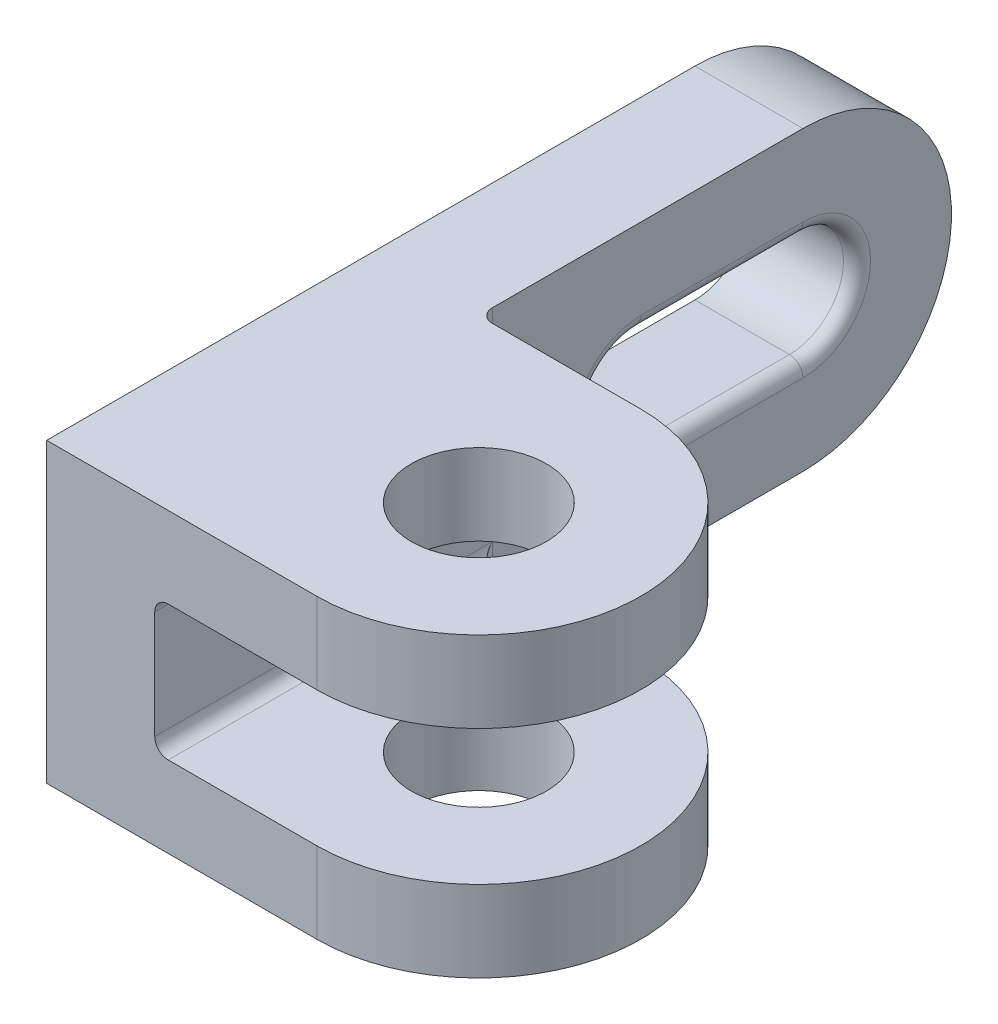
ISO-10303-21;
HEADER;
FILE_DESCRIPTION(('STEP AP214'),'2;1');
FILE_NAME('part.step','',(''),(''),'','','');
FILE_SCHEMA(('AUTOMOTIVE_DESIGN { 1 0 10303 214 1 1 1 1 }'));
ENDSEC;
DATA;
#1=APPLICATION_CONTEXT('core data for automotive mechanical design processes');
#2=APPLICATION_PROTOCOL_DEFINITION('international standard','automotive_design',2000,#1);
#3=PRODUCT_CONTEXT('',#1,'mechanical');
#4=PRODUCT('Part','Part','',(#3));
#5=PRODUCT_RELATED_PRODUCT_CATEGORY('part','',(#4));
#6=PRODUCT_DEFINITION_FORMATION('','',#4);
#7=PRODUCT_DEFINITION_CONTEXT('part definition',#1,'design');
#8=PRODUCT_DEFINITION('design','',#6,#7);
#9=PRODUCT_DEFINITION_SHAPE('','',#8);
#10=(LENGTH_UNIT() NAMED_UNIT(*) SI_UNIT(.MILLI.,.METRE.));
#11=(NAMED_UNIT(*) PLANE_ANGLE_UNIT() SI_UNIT($,.RADIAN.));
#12=(NAMED_UNIT(*) SI_UNIT($,.STERADIAN.) SOLID_ANGLE_UNIT());
#13=UNCERTAINTY_MEASURE_WITH_UNIT(LENGTH_MEASURE(1.E-05),#10,'distance_accuracy_value','');
#14=(GEOMETRIC_REPRESENTATION_CONTEXT(3) GLOBAL_UNCERTAINTY_ASSIGNED_CONTEXT((#13)) GLOBAL_UNIT_ASSIGNED_CONTEXT((#10,
#11,#12)) REPRESENTATION_CONTEXT('',''));
#15=CARTESIAN_POINT('',(0.,0.,0.));
#16=DIRECTION('',(0.,0.,1.));
#17=DIRECTION('',(1.,0.,0.));
#18=AXIS2_PLACEMENT_3D('',#15,#16,#17);
#19=CARTESIAN_POINT('',(16.,0.,-96.));
#20=DIRECTION('',(0.,1.,0.));
#21=DIRECTION('',(0.,0.,1.));
#22=AXIS2_PLACEMENT_3D('',#19,#20,#21);
#23=PLANE('',#22);
#24=CARTESIAN_POINT('',(40.,0.,-24.));
#25=DIRECTION('',(0.,-1.,0.));
#26=DIRECTION('',(0.,0.,-1.));
#27=AXIS2_PLACEMENT_3D('',#24,#25,#26);
#28=CIRCLE('',#27,10.);
#29=CARTESIAN_POINT('',(40.,0.,-34.));
#30=VERTEX_POINT('',#29);
#31=EDGE_CURVE('E308',#30,#30,#28,.T.);
#32=ORIENTED_EDGE('',*,*,#31,.F.);
#33=EDGE_LOOP('',(#32));
#34=FACE_BOUND('',#33,.T.);
#35=DIRECTION('',(0.,0.,-1.));
#36=VECTOR('',#35,1.);
#37=CARTESIAN_POINT('',(16.,0.,-96.));
#38=LINE('',#37,#36);
#39=CARTESIAN_POINT('',(16.,0.,-50.));
#40=VERTEX_POINT('',#39);
#41=CARTESIAN_POINT('',(16.,0.,-96.));
#42=VERTEX_POINT('',#41);
#43=EDGE_CURVE('E250',#40,#42,#38,.T.);
#44=ORIENTED_EDGE('',*,*,#43,.F.);
#45=CARTESIAN_POINT('',(18.,0.,-50.));
#46=DIRECTION('',(0.,1.,0.));
#47=DIRECTION('',(0.,0.,1.));
#48=AXIS2_PLACEMENT_3D('',#45,#46,#47);
#49=CIRCLE('',#48,2.);
#50=CARTESIAN_POINT('',(18.,0.,-48.));
#51=VERTEX_POINT('',#50);
#52=EDGE_CURVE('E282',#40,#51,#49,.T.);
#53=ORIENTED_EDGE('',*,*,#52,.T.);
#54=DIRECTION('',(1.,0.,0.));
#55=VECTOR('',#54,1.);
#56=CARTESIAN_POINT('',(40.,0.,-48.));
#57=LINE('',#56,#55);
#58=CARTESIAN_POINT('',(40.,0.,-48.));
#59=VERTEX_POINT('',#58);
#60=EDGE_CURVE('E202',#51,#59,#57,.T.);
#61=ORIENTED_EDGE('',*,*,#60,.T.);
#62=CARTESIAN_POINT('',(40.,0.,-24.));
#63=DIRECTION('',(0.,-1.,0.));
#64=DIRECTION('',(0.,0.,1.));
#65=AXIS2_PLACEMENT_3D('',#62,#63,#64);
#66=CIRCLE('',#65,24.);
#67=CARTESIAN_POINT('',(40.,0.,0.));
#68=VERTEX_POINT('',#67);
#69=EDGE_CURVE('E209',#59,#68,#66,.T.);
#70=ORIENTED_EDGE('',*,*,#69,.T.);
#71=DIRECTION('',(-1.,0.,0.));
#72=VECTOR('',#71,1.);
#73=CARTESIAN_POINT('',(16.,0.,0.));
#74=LINE('',#73,#72);
#75=CARTESIAN_POINT('',(0.,0.,0.));
#76=VERTEX_POINT('',#75);
#77=EDGE_CURVE('E256',#68,#76,#74,.T.);
#78=ORIENTED_EDGE('',*,*,#77,.T.);
#79=DIRECTION('',(0.,0.,-1.));
#80=VECTOR('',#79,1.);
#81=CARTESIAN_POINT('',(0.,0.,-96.));
#82=LINE('',#81,#80);
#83=CARTESIAN_POINT('',(0.,0.,-96.));
#84=VERTEX_POINT('',#83);
#85=EDGE_CURVE('E238',#76,#84,#82,.T.);
#86=ORIENTED_EDGE('',*,*,#85,.T.);
#87=DIRECTION('',(-1.,0.,0.));
#88=VECTOR('',#87,1.);
#89=CARTESIAN_POINT('',(16.,0.,-96.));
#90=LINE('',#89,#88);
#91=EDGE_CURVE('E275',#42,#84,#90,.T.);
#92=ORIENTED_EDGE('',*,*,#91,.F.);
#93=EDGE_LOOP('',(#44,#53,#61,#70,#78,#86,#92));
#94=FACE_BOUND('',#93,.T.);
#95=ADVANCED_FACE('F39',(#34,#94),#23,.F.);
#96=CARTESIAN_POINT('',(16.,22.,-96.));
#97=DIRECTION('',(-1.,0.,0.));
#98=DIRECTION('',(0.,0.,1.));
#99=AXIS2_PLACEMENT_3D('',#96,#97,#98);
#100=CYLINDRICAL_SURFACE('',#99,22.);
#101=CARTESIAN_POINT('',(0.,22.,-96.));
#102=DIRECTION('',(1.,0.,0.));
#103=DIRECTION('',(0.,0.,1.));
#104=AXIS2_PLACEMENT_3D('',#101,#102,#103);
#105=CIRCLE('',#104,22.);
#106=CARTESIAN_POINT('',(0.,44.,-96.));
#107=VERTEX_POINT('',#106);
#108=EDGE_CURVE('E257',#84,#107,#105,.T.);
#109=ORIENTED_EDGE('',*,*,#108,.T.);
#110=DIRECTION('',(-1.,0.,0.));
#111=VECTOR('',#110,1.);
#112=CARTESIAN_POINT('',(16.,44.,-96.));
#113=LINE('',#112,#111);
#114=CARTESIAN_POINT('',(16.,44.,-96.));
#115=VERTEX_POINT('',#114);
#116=EDGE_CURVE('E267',#115,#107,#113,.T.);
#117=ORIENTED_EDGE('',*,*,#116,.F.);
#118=CARTESIAN_POINT('',(16.,22.,-96.));
#119=DIRECTION('',(1.,0.,0.));
#120=DIRECTION('',(0.,0.,1.));
#121=AXIS2_PLACEMENT_3D('',#118,#119,#120);
#122=CIRCLE('',#121,22.);
#123=EDGE_CURVE('E247',#42,#115,#122,.T.);
#124=ORIENTED_EDGE('',*,*,#123,.F.);
#125=ORIENTED_EDGE('',*,*,#91,.T.);
#126=EDGE_LOOP('',(#109,#117,#124,#125));
#127=FACE_BOUND('',#126,.T.);
#128=ADVANCED_FACE('F375',(#127),#100,.T.);
#129=CARTESIAN_POINT('',(16.,44.,0.));
#130=DIRECTION('',(0.,-1.,0.));
#131=DIRECTION('',(0.,0.,-1.));
#132=AXIS2_PLACEMENT_3D('',#129,#130,#131);
#133=PLANE('',#132);
#134=CARTESIAN_POINT('',(40.,44.,-24.));
#135=DIRECTION('',(0.,1.,0.));
#136=DIRECTION('',(0.,0.,1.));
#137=AXIS2_PLACEMENT_3D('',#134,#135,#136);
#138=CIRCLE('',#137,10.);
#139=CARTESIAN_POINT('',(40.,44.,-14.));
#140=VERTEX_POINT('',#139);
#141=EDGE_CURVE('E608',#140,#140,#138,.T.);
#142=ORIENTED_EDGE('',*,*,#141,.F.);
#143=EDGE_LOOP('',(#142));
#144=FACE_BOUND('',#143,.T.);
#145=DIRECTION('',(0.,0.,1.));
#146=VECTOR('',#145,1.);
#147=CARTESIAN_POINT('',(0.,44.,0.));
#148=LINE('',#147,#146);
#149=CARTESIAN_POINT('',(0.,44.,0.));
#150=VERTEX_POINT('',#149);
#151=EDGE_CURVE('E265',#107,#150,#148,.T.);
#152=ORIENTED_EDGE('',*,*,#151,.T.);
#153=DIRECTION('',(-1.,0.,0.));
#154=VECTOR('',#153,1.);
#155=CARTESIAN_POINT('',(16.,44.,0.));
#156=LINE('',#155,#154);
#157=CARTESIAN_POINT('',(40.,44.,0.));
#158=VERTEX_POINT('',#157);
#159=EDGE_CURVE('E270',#158,#150,#156,.T.);
#160=ORIENTED_EDGE('',*,*,#159,.F.);
#161=CARTESIAN_POINT('',(40.,44.,-24.));
#162=DIRECTION('',(0.,1.,0.));
#163=DIRECTION('',(0.,0.,1.));
#164=AXIS2_PLACEMENT_3D('',#161,#162,#163);
#165=CIRCLE('',#164,24.);
#166=CARTESIAN_POINT('',(39.9999999999999,44.,-48.));
#167=VERTEX_POINT('',#166);
#168=EDGE_CURVE('E191',#158,#167,#165,.T.);
#169=ORIENTED_EDGE('',*,*,#168,.T.);
#170=DIRECTION('',(-1.,0.,0.));
#171=VECTOR('',#170,1.);
#172=CARTESIAN_POINT('',(39.9999999999999,44.,-48.));
#173=LINE('',#172,#171);
#174=CARTESIAN_POINT('',(18.,44.,-48.));
#175=VERTEX_POINT('',#174);
#176=EDGE_CURVE('E184',#167,#175,#173,.T.);
#177=ORIENTED_EDGE('',*,*,#176,.T.);
#178=CARTESIAN_POINT('',(18.,44.,-50.));
#179=DIRECTION('',(0.,-1.,0.));
#180=DIRECTION('',(0.,0.,-1.));
#181=AXIS2_PLACEMENT_3D('',#178,#179,#180);
#182=CIRCLE('',#181,2.);
#183=CARTESIAN_POINT('',(16.,44.,-50.));
#184=VERTEX_POINT('',#183);
#185=EDGE_CURVE('E301',#175,#184,#182,.T.);
#186=ORIENTED_EDGE('',*,*,#185,.T.);
#187=DIRECTION('',(0.,0.,1.));
#188=VECTOR('',#187,1.);
#189=CARTESIAN_POINT('',(16.,44.,0.));
#190=LINE('',#189,#188);
#191=EDGE_CURVE('E252',#115,#184,#190,.T.);
#192=ORIENTED_EDGE('',*,*,#191,.F.);
#193=ORIENTED_EDGE('',*,*,#116,.T.);
#194=EDGE_LOOP('',(#152,#160,#169,#177,#186,#192,#193));
#195=FACE_BOUND('',#194,.T.);
#196=ADVANCED_FACE('F379',(#144,#195),#133,.F.);
#197=CARTESIAN_POINT('',(16.,0.,0.));
#198=DIRECTION('',(0.,0.,-1.));
#199=DIRECTION('',(-1.,0.,0.));
#200=AXIS2_PLACEMENT_3D('',#197,#198,#199);
#201=PLANE('',#200);
#202=DIRECTION('',(0.,-1.,0.));
#203=VECTOR('',#202,1.);
#204=CARTESIAN_POINT('',(0.,0.,0.));
#205=LINE('',#204,#203);
#206=EDGE_CURVE('E249',#150,#76,#205,.T.);
#207=ORIENTED_EDGE('',*,*,#206,.T.);
#208=ORIENTED_EDGE('',*,*,#77,.F.);
#209=DIRECTION('',(0.,-1.,0.));
#210=VECTOR('',#209,1.);
#211=CARTESIAN_POINT('',(40.,12.,0.));
#212=LINE('',#211,#210);
#213=CARTESIAN_POINT('',(40.,12.,0.));
#214=VERTEX_POINT('',#213);
#215=EDGE_CURVE('E219',#214,#68,#212,.T.);
#216=ORIENTED_EDGE('',*,*,#215,.F.);
#217=DIRECTION('',(-1.,0.,0.));
#218=VECTOR('',#217,1.);
#219=CARTESIAN_POINT('',(0.,12.,0.));
#220=LINE('',#219,#218);
#221=CARTESIAN_POINT('',(18.,12.,0.));
#222=VERTEX_POINT('',#221);
#223=EDGE_CURVE('E213',#214,#222,#220,.T.);
#224=ORIENTED_EDGE('',*,*,#223,.T.);
#225=CARTESIAN_POINT('',(18.,14.,0.));
#226=DIRECTION('',(0.,0.,-1.));
#227=DIRECTION('',(-1.,0.,0.));
#228=AXIS2_PLACEMENT_3D('',#225,#226,#227);
#229=CIRCLE('',#228,2.);
#230=CARTESIAN_POINT('',(16.,14.,0.));
#231=VERTEX_POINT('',#230);
#232=EDGE_CURVE('E298',#222,#231,#229,.T.);
#233=ORIENTED_EDGE('',*,*,#232,.T.);
#234=DIRECTION('',(0.,-1.,0.));
#235=VECTOR('',#234,1.);
#236=CARTESIAN_POINT('',(16.,0.,0.));
#237=LINE('',#236,#235);
#238=CARTESIAN_POINT('',(16.,30.,0.));
#239=VERTEX_POINT('',#238);
#240=EDGE_CURVE('E254',#239,#231,#237,.T.);
#241=ORIENTED_EDGE('',*,*,#240,.F.);
#242=CARTESIAN_POINT('',(18.,30.,0.));
#243=DIRECTION('',(0.,0.,-1.));
#244=DIRECTION('',(-1.,0.,0.));
#245=AXIS2_PLACEMENT_3D('',#242,#243,#244);
#246=CIRCLE('',#245,2.);
#247=CARTESIAN_POINT('',(18.,32.,0.));
#248=VERTEX_POINT('',#247);
#249=EDGE_CURVE('E178',#239,#248,#246,.T.);
#250=ORIENTED_EDGE('',*,*,#249,.T.);
#251=DIRECTION('',(1.,0.,0.));
#252=VECTOR('',#251,1.);
#253=CARTESIAN_POINT('',(0.,32.,0.));
#254=LINE('',#253,#252);
#255=CARTESIAN_POINT('',(40.,32.,0.));
#256=VERTEX_POINT('',#255);
#257=EDGE_CURVE('E168',#248,#256,#254,.T.);
#258=ORIENTED_EDGE('',*,*,#257,.T.);
#259=DIRECTION('',(0.,1.,0.));
#260=VECTOR('',#259,1.);
#261=CARTESIAN_POINT('',(40.,32.,0.));
#262=LINE('',#261,#260);
#263=EDGE_CURVE('E174',#256,#158,#262,.T.);
#264=ORIENTED_EDGE('',*,*,#263,.T.);
#265=ORIENTED_EDGE('',*,*,#159,.T.);
#266=EDGE_LOOP('',(#207,#208,#216,#224,#233,#241,#250,#258,#264,#265));
#267=FACE_BOUND('',#266,.T.);
#268=ADVANCED_FACE('F175',(#267),#201,.F.);
#269=CARTESIAN_POINT('',(16.,22.,-96.));
#270=DIRECTION('',(-1.,0.,0.));
#271=DIRECTION('',(0.,0.,1.));
#272=AXIS2_PLACEMENT_3D('',#269,#270,#271);
#273=PLANE('',#272);
#274=DIRECTION('',(0.,0.,1.));
#275=VECTOR('',#274,1.);
#276=CARTESIAN_POINT('',(16.,32.,-96.));
#277=LINE('',#276,#275);
#278=CARTESIAN_POINT('',(16.,32.,-72.));
#279=VERTEX_POINT('',#278);
#280=CARTESIAN_POINT('',(16.,32.,-96.));
#281=VERTEX_POINT('',#280);
#282=EDGE_CURVE('E310',#279,#281,#277,.F.);
#283=ORIENTED_EDGE('',*,*,#282,.T.);
#284=CARTESIAN_POINT('',(16.,22.,-96.));
#285=DIRECTION('',(-1.,0.,0.));
#286=DIRECTION('',(0.,0.,1.));
#287=AXIS2_PLACEMENT_3D('',#284,#285,#286);
#288=CIRCLE('',#287,10.);
#289=CARTESIAN_POINT('',(16.,12.,-96.));
#290=VERTEX_POINT('',#289);
#291=EDGE_CURVE('E312',#281,#290,#288,.T.);
#292=ORIENTED_EDGE('',*,*,#291,.T.);
#293=DIRECTION('',(0.,0.,-1.));
#294=VECTOR('',#293,1.);
#295=CARTESIAN_POINT('',(16.,12.,-96.));
#296=LINE('',#295,#294);
#297=CARTESIAN_POINT('',(16.,12.,-72.));
#298=VERTEX_POINT('',#297);
#299=EDGE_CURVE('E311',#290,#298,#296,.F.);
#300=ORIENTED_EDGE('',*,*,#299,.T.);
#301=CARTESIAN_POINT('',(16.,22.,-72.));
#302=DIRECTION('',(-1.,0.,0.));
#303=DIRECTION('',(0.,0.,1.));
#304=AXIS2_PLACEMENT_3D('',#301,#302,#303);
#305=CIRCLE('',#304,10.);
#306=EDGE_CURVE('E313',#298,#279,#305,.T.);
#307=ORIENTED_EDGE('',*,*,#306,.T.);
#308=EDGE_LOOP('',(#283,#292,#300,#307));
#309=FACE_BOUND('',#308,.T.);
#310=ORIENTED_EDGE('',*,*,#240,.T.);
#311=DIRECTION('',(0.,0.,-1.));
#312=VECTOR('',#311,1.);
#313=CARTESIAN_POINT('',(16.,14.,-96.));
#314=LINE('',#313,#312);
#315=CARTESIAN_POINT('',(16.,14.,-50.));
#316=VERTEX_POINT('',#315);
#317=EDGE_CURVE('E290',#231,#316,#314,.T.);
#318=ORIENTED_EDGE('',*,*,#317,.T.);
#319=DIRECTION('',(0.,-1.,0.));
#320=VECTOR('',#319,1.);
#321=CARTESIAN_POINT('',(16.,22.,-50.));
#322=LINE('',#321,#320);
#323=EDGE_CURVE('E274',#316,#40,#322,.T.);
#324=ORIENTED_EDGE('',*,*,#323,.T.);
#325=ORIENTED_EDGE('',*,*,#43,.T.);
#326=ORIENTED_EDGE('',*,*,#123,.T.);
#327=ORIENTED_EDGE('',*,*,#191,.T.);
#328=DIRECTION('',(0.,-1.,0.));
#329=VECTOR('',#328,1.);
#330=CARTESIAN_POINT('',(16.,22.,-50.));
#331=LINE('',#330,#329);
#332=CARTESIAN_POINT('',(16.,30.,-50.));
#333=VERTEX_POINT('',#332);
#334=EDGE_CURVE('E283',#184,#333,#331,.T.);
#335=ORIENTED_EDGE('',*,*,#334,.T.);
#336=DIRECTION('',(0.,0.,-1.));
#337=VECTOR('',#336,1.);
#338=CARTESIAN_POINT('',(16.,30.,0.));
#339=LINE('',#338,#337);
#340=EDGE_CURVE('E281',#333,#239,#339,.F.);
#341=ORIENTED_EDGE('',*,*,#340,.T.);
#342=EDGE_LOOP('',(#310,#318,#324,#325,#326,#327,#335,#341));
#343=FACE_BOUND('',#342,.T.);
#344=ADVANCED_FACE('F339',(#309,#343),#273,.F.);
#345=CARTESIAN_POINT('',(0.,22.,-96.));
#346=DIRECTION('',(-1.,0.,0.));
#347=DIRECTION('',(0.,0.,1.));
#348=AXIS2_PLACEMENT_3D('',#345,#346,#347);
#349=PLANE('',#348);
#350=ORIENTED_EDGE('',*,*,#206,.F.);
#351=ORIENTED_EDGE('',*,*,#151,.F.);
#352=ORIENTED_EDGE('',*,*,#108,.F.);
#353=ORIENTED_EDGE('',*,*,#85,.F.);
#354=EDGE_LOOP('',(#350,#351,#352,#353));
#355=FACE_BOUND('',#354,.T.);
#356=CARTESIAN_POINT('',(0.,22.,-72.));
#357=DIRECTION('',(1.,0.,0.));
#358=DIRECTION('',(0.,0.,-1.));
#359=AXIS2_PLACEMENT_3D('',#356,#357,#358);
#360=CIRCLE('',#359,8.00000000000001);
#361=CARTESIAN_POINT('',(0.,30.,-72.));
#362=VERTEX_POINT('',#361);
#363=CARTESIAN_POINT('',(0.,14.,-72.));
#364=VERTEX_POINT('',#363);
#365=EDGE_CURVE('E224',#362,#364,#360,.T.);
#366=ORIENTED_EDGE('',*,*,#365,.T.);
#367=DIRECTION('',(0.,0.,-1.));
#368=VECTOR('',#367,1.);
#369=CARTESIAN_POINT('',(0.,14.,-96.));
#370=LINE('',#369,#368);
#371=CARTESIAN_POINT('',(0.,14.,-96.));
#372=VERTEX_POINT('',#371);
#373=EDGE_CURVE('E228',#364,#372,#370,.T.);
#374=ORIENTED_EDGE('',*,*,#373,.T.);
#375=CARTESIAN_POINT('',(0.,22.,-96.));
#376=DIRECTION('',(1.,0.,0.));
#377=DIRECTION('',(0.,0.,-1.));
#378=AXIS2_PLACEMENT_3D('',#375,#376,#377);
#379=CIRCLE('',#378,8.00000000000001);
#380=CARTESIAN_POINT('',(0.,30.,-96.));
#381=VERTEX_POINT('',#380);
#382=EDGE_CURVE('E231',#372,#381,#379,.T.);
#383=ORIENTED_EDGE('',*,*,#382,.T.);
#384=DIRECTION('',(0.,0.,1.));
#385=VECTOR('',#384,1.);
#386=CARTESIAN_POINT('',(0.,30.,-72.));
#387=LINE('',#386,#385);
#388=EDGE_CURVE('E232',#381,#362,#387,.T.);
#389=ORIENTED_EDGE('',*,*,#388,.T.);
#390=EDGE_LOOP('',(#366,#374,#383,#389));
#391=FACE_BOUND('',#390,.T.);
#392=ADVANCED_FACE('F354',(#355,#391),#349,.T.);
#393=CARTESIAN_POINT('',(0.,22.,-72.));
#394=DIRECTION('',(1.,0.,0.));
#395=DIRECTION('',(0.,0.,-1.));
#396=AXIS2_PLACEMENT_3D('',#393,#394,#395);
#397=CYLINDRICAL_SURFACE('',#396,8.00000000000001);
#398=DIRECTION('',(1.,0.,0.));
#399=VECTOR('',#398,1.);
#400=CARTESIAN_POINT('',(0.,30.,-72.));
#401=LINE('',#400,#399);
#402=CARTESIAN_POINT('',(14.,30.,-72.));
#403=VERTEX_POINT('',#402);
#404=EDGE_CURVE('E236',#362,#403,#401,.T.);
#405=ORIENTED_EDGE('',*,*,#404,.T.);
#406=CARTESIAN_POINT('',(14.,22.,-72.));
#407=DIRECTION('',(-1.,0.,0.));
#408=DIRECTION('',(0.,0.,1.));
#409=AXIS2_PLACEMENT_3D('',#406,#407,#408);
#410=CIRCLE('',#409,8.00000000000001);
#411=CARTESIAN_POINT('',(14.,14.,-72.));
#412=VERTEX_POINT('',#411);
#413=EDGE_CURVE('E48',#403,#412,#410,.F.);
#414=ORIENTED_EDGE('',*,*,#413,.T.);
#415=DIRECTION('',(1.,0.,0.));
#416=VECTOR('',#415,1.);
#417=CARTESIAN_POINT('',(0.,14.,-72.));
#418=LINE('',#417,#416);
#419=EDGE_CURVE('E240',#364,#412,#418,.T.);
#420=ORIENTED_EDGE('',*,*,#419,.F.);
#421=ORIENTED_EDGE('',*,*,#365,.F.);
#422=EDGE_LOOP('',(#405,#414,#420,#421));
#423=FACE_BOUND('',#422,.T.);
#424=ADVANCED_FACE('F358',(#423),#397,.F.);
#425=CARTESIAN_POINT('',(0.,30.,-72.));
#426=DIRECTION('',(0.,1.,0.));
#427=DIRECTION('',(0.,0.,1.));
#428=AXIS2_PLACEMENT_3D('',#425,#426,#427);
#429=PLANE('',#428);
#430=DIRECTION('',(1.,0.,0.));
#431=VECTOR('',#430,1.);
#432=CARTESIAN_POINT('',(0.,30.,-96.));
#433=LINE('',#432,#431);
#434=CARTESIAN_POINT('',(14.,30.,-96.));
#435=VERTEX_POINT('',#434);
#436=EDGE_CURVE('E242',#381,#435,#433,.T.);
#437=ORIENTED_EDGE('',*,*,#436,.T.);
#438=DIRECTION('',(0.,0.,1.));
#439=VECTOR('',#438,1.);
#440=CARTESIAN_POINT('',(14.,30.,-72.));
#441=LINE('',#440,#439);
#442=EDGE_CURVE('E11',#435,#403,#441,.T.);
#443=ORIENTED_EDGE('',*,*,#442,.T.);
#444=ORIENTED_EDGE('',*,*,#404,.F.);
#445=ORIENTED_EDGE('',*,*,#388,.F.);
#446=EDGE_LOOP('',(#437,#443,#444,#445));
#447=FACE_BOUND('',#446,.T.);
#448=ADVANCED_FACE('F352',(#447),#429,.F.);
#449=CARTESIAN_POINT('',(0.,22.,-96.));
#450=DIRECTION('',(1.,0.,0.));
#451=DIRECTION('',(0.,0.,-1.));
#452=AXIS2_PLACEMENT_3D('',#449,#450,#451);
#453=CYLINDRICAL_SURFACE('',#452,8.00000000000001);
#454=DIRECTION('',(1.,0.,0.));
#455=VECTOR('',#454,1.);
#456=CARTESIAN_POINT('',(0.,14.,-96.));
#457=LINE('',#456,#455);
#458=CARTESIAN_POINT('',(14.,14.,-96.));
#459=VERTEX_POINT('',#458);
#460=EDGE_CURVE('E243',#372,#459,#457,.T.);
#461=ORIENTED_EDGE('',*,*,#460,.T.);
#462=CARTESIAN_POINT('',(14.,22.,-96.));
#463=DIRECTION('',(-1.,0.,0.));
#464=DIRECTION('',(0.,0.,1.));
#465=AXIS2_PLACEMENT_3D('',#462,#463,#464);
#466=CIRCLE('',#465,8.00000000000001);
#467=EDGE_CURVE('E303',#459,#435,#466,.F.);
#468=ORIENTED_EDGE('',*,*,#467,.T.);
#469=ORIENTED_EDGE('',*,*,#436,.F.);
#470=ORIENTED_EDGE('',*,*,#382,.F.);
#471=EDGE_LOOP('',(#461,#468,#469,#470));
#472=FACE_BOUND('',#471,.T.);
#473=ADVANCED_FACE('F346',(#472),#453,.F.);
#474=CARTESIAN_POINT('',(0.,14.,-96.));
#475=DIRECTION('',(0.,-1.,0.));
#476=DIRECTION('',(0.,0.,-1.));
#477=AXIS2_PLACEMENT_3D('',#474,#475,#476);
#478=PLANE('',#477);
#479=ORIENTED_EDGE('',*,*,#419,.T.);
#480=DIRECTION('',(0.,0.,-1.));
#481=VECTOR('',#480,1.);
#482=CARTESIAN_POINT('',(14.,14.,-96.));
#483=LINE('',#482,#481);
#484=EDGE_CURVE('E318',#412,#459,#483,.T.);
#485=ORIENTED_EDGE('',*,*,#484,.T.);
#486=ORIENTED_EDGE('',*,*,#460,.F.);
#487=ORIENTED_EDGE('',*,*,#373,.F.);
#488=EDGE_LOOP('',(#479,#485,#486,#487));
#489=FACE_BOUND('',#488,.T.);
#490=ADVANCED_FACE('F360',(#489),#478,.F.);
#491=CARTESIAN_POINT('',(40.,12.,-48.));
#492=DIRECTION('',(0.,0.,-1.));
#493=DIRECTION('',(-1.,0.,0.));
#494=AXIS2_PLACEMENT_3D('',#491,#492,#493);
#495=PLANE('',#494);
#496=ORIENTED_EDGE('',*,*,#60,.F.);
#497=DIRECTION('',(0.,-1.,0.));
#498=VECTOR('',#497,1.);
#499=CARTESIAN_POINT('',(18.,12.,-48.));
#500=LINE('',#499,#498);
#501=CARTESIAN_POINT('',(18.,12.,-48.));
#502=VERTEX_POINT('',#501);
#503=EDGE_CURVE('E279',#51,#502,#500,.F.);
#504=ORIENTED_EDGE('',*,*,#503,.T.);
#505=DIRECTION('',(1.,0.,0.));
#506=VECTOR('',#505,1.);
#507=CARTESIAN_POINT('',(40.,12.,-48.));
#508=LINE('',#507,#506);
#509=CARTESIAN_POINT('',(40.,12.,-48.));
#510=VERTEX_POINT('',#509);
#511=EDGE_CURVE('E210',#502,#510,#508,.T.);
#512=ORIENTED_EDGE('',*,*,#511,.T.);
#513=DIRECTION('',(0.,-1.,0.));
#514=VECTOR('',#513,1.);
#515=CARTESIAN_POINT('',(40.,12.,-48.));
#516=LINE('',#515,#514);
#517=EDGE_CURVE('E216',#510,#59,#516,.T.);
#518=ORIENTED_EDGE('',*,*,#517,.T.);
#519=EDGE_LOOP('',(#496,#504,#512,#518));
#520=FACE_BOUND('',#519,.T.);
#521=ADVANCED_FACE('F423',(#520),#495,.T.);
#522=CARTESIAN_POINT('',(40.,12.,-24.));
#523=DIRECTION('',(0.,1.,0.));
#524=DIRECTION('',(0.,0.,1.));
#525=AXIS2_PLACEMENT_3D('',#522,#523,#524);
#526=PLANE('',#525);
#527=CARTESIAN_POINT('',(40.,12.,-24.));
#528=DIRECTION('',(0.,-1.,0.));
#529=DIRECTION('',(0.,0.,-1.));
#530=AXIS2_PLACEMENT_3D('',#527,#528,#529);
#531=CIRCLE('',#530,10.);
#532=CARTESIAN_POINT('',(40.,12.,-34.));
#533=VERTEX_POINT('',#532);
#534=EDGE_CURVE('E610',#533,#533,#531,.T.);
#535=ORIENTED_EDGE('',*,*,#534,.T.);
#536=EDGE_LOOP('',(#535));
#537=FACE_BOUND('',#536,.T.);
#538=ORIENTED_EDGE('',*,*,#511,.F.);
#539=DIRECTION('',(0.,0.,-1.));
#540=VECTOR('',#539,1.);
#541=CARTESIAN_POINT('',(18.,12.,-24.));
#542=LINE('',#541,#540);
#543=EDGE_CURVE('E289',#502,#222,#542,.F.);
#544=ORIENTED_EDGE('',*,*,#543,.T.);
#545=ORIENTED_EDGE('',*,*,#223,.F.);
#546=CARTESIAN_POINT('',(40.,12.,-24.));
#547=DIRECTION('',(0.,-1.,0.));
#548=DIRECTION('',(0.,0.,1.));
#549=AXIS2_PLACEMENT_3D('',#546,#547,#548);
#550=CIRCLE('',#549,24.);
#551=EDGE_CURVE('E207',#510,#214,#550,.T.);
#552=ORIENTED_EDGE('',*,*,#551,.F.);
#553=EDGE_LOOP('',(#538,#544,#545,#552));
#554=FACE_BOUND('',#553,.T.);
#555=ADVANCED_FACE('F492',(#537,#554),#526,.T.);
#556=CARTESIAN_POINT('',(40.,12.,-24.));
#557=DIRECTION('',(0.,-1.,0.));
#558=DIRECTION('',(0.,0.,-1.));
#559=AXIS2_PLACEMENT_3D('',#556,#557,#558);
#560=CYLINDRICAL_SURFACE('',#559,24.);
#561=ORIENTED_EDGE('',*,*,#69,.F.);
#562=ORIENTED_EDGE('',*,*,#517,.F.);
#563=ORIENTED_EDGE('',*,*,#551,.T.);
#564=ORIENTED_EDGE('',*,*,#215,.T.);
#565=EDGE_LOOP('',(#561,#562,#563,#564));
#566=FACE_BOUND('',#565,.T.);
#567=ADVANCED_FACE('F489',(#566),#560,.T.);
#568=CARTESIAN_POINT('',(39.9999999999999,32.,-48.));
#569=DIRECTION('',(0.,0.,-1.));
#570=DIRECTION('',(-1.,0.,0.));
#571=AXIS2_PLACEMENT_3D('',#568,#569,#570);
#572=PLANE('',#571);
#573=DIRECTION('',(-1.,0.,0.));
#574=VECTOR('',#573,1.);
#575=CARTESIAN_POINT('',(39.9999999999999,32.,-48.));
#576=LINE('',#575,#574);
#577=CARTESIAN_POINT('',(39.9999999999999,32.,-48.));
#578=VERTEX_POINT('',#577);
#579=CARTESIAN_POINT('',(18.,32.,-48.));
#580=VERTEX_POINT('',#579);
#581=EDGE_CURVE('E193',#578,#580,#576,.T.);
#582=ORIENTED_EDGE('',*,*,#581,.T.);
#583=DIRECTION('',(0.,-1.,0.));
#584=VECTOR('',#583,1.);
#585=CARTESIAN_POINT('',(18.,32.,-48.));
#586=LINE('',#585,#584);
#587=EDGE_CURVE('E294',#580,#175,#586,.F.);
#588=ORIENTED_EDGE('',*,*,#587,.T.);
#589=ORIENTED_EDGE('',*,*,#176,.F.);
#590=DIRECTION('',(0.,1.,0.));
#591=VECTOR('',#590,1.);
#592=CARTESIAN_POINT('',(39.9999999999999,32.,-48.));
#593=LINE('',#592,#591);
#594=EDGE_CURVE('E195',#578,#167,#593,.T.);
#595=ORIENTED_EDGE('',*,*,#594,.F.);
#596=EDGE_LOOP('',(#582,#588,#589,#595));
#597=FACE_BOUND('',#596,.T.);
#598=ADVANCED_FACE('F495',(#597),#572,.T.);
#599=CARTESIAN_POINT('',(40.,32.,-24.));
#600=DIRECTION('',(0.,1.,0.));
#601=DIRECTION('',(0.,0.,1.));
#602=AXIS2_PLACEMENT_3D('',#599,#600,#601);
#603=PLANE('',#602);
#604=CARTESIAN_POINT('',(40.,32.,-24.));
#605=DIRECTION('',(0.,1.,0.));
#606=DIRECTION('',(0.,0.,1.));
#607=AXIS2_PLACEMENT_3D('',#604,#605,#606);
#608=CIRCLE('',#607,10.);
#609=CARTESIAN_POINT('',(40.,32.,-14.));
#610=VERTEX_POINT('',#609);
#611=EDGE_CURVE('E205',#610,#610,#608,.T.);
#612=ORIENTED_EDGE('',*,*,#611,.T.);
#613=EDGE_LOOP('',(#612));
#614=FACE_BOUND('',#613,.T.);
#615=ORIENTED_EDGE('',*,*,#257,.F.);
#616=DIRECTION('',(0.,0.,-1.));
#617=VECTOR('',#616,1.);
#618=CARTESIAN_POINT('',(18.,32.,-48.));
#619=LINE('',#618,#617);
#620=EDGE_CURVE('E295',#248,#580,#619,.T.);
#621=ORIENTED_EDGE('',*,*,#620,.T.);
#622=ORIENTED_EDGE('',*,*,#581,.F.);
#623=CARTESIAN_POINT('',(40.,32.,-24.));
#624=DIRECTION('',(0.,1.,0.));
#625=DIRECTION('',(0.,0.,1.));
#626=AXIS2_PLACEMENT_3D('',#623,#624,#625);
#627=CIRCLE('',#626,24.);
#628=EDGE_CURVE('E181',#256,#578,#627,.T.);
#629=ORIENTED_EDGE('',*,*,#628,.F.);
#630=EDGE_LOOP('',(#615,#621,#622,#629));
#631=FACE_BOUND('',#630,.T.);
#632=ADVANCED_FACE('F194',(#614,#631),#603,.F.);
#633=CARTESIAN_POINT('',(40.,32.,-24.));
#634=DIRECTION('',(0.,1.,0.));
#635=DIRECTION('',(0.,0.,1.));
#636=AXIS2_PLACEMENT_3D('',#633,#634,#635);
#637=CYLINDRICAL_SURFACE('',#636,24.);
#638=ORIENTED_EDGE('',*,*,#168,.F.);
#639=ORIENTED_EDGE('',*,*,#263,.F.);
#640=ORIENTED_EDGE('',*,*,#628,.T.);
#641=ORIENTED_EDGE('',*,*,#594,.T.);
#642=EDGE_LOOP('',(#638,#639,#640,#641));
#643=FACE_BOUND('',#642,.T.);
#644=ADVANCED_FACE('F188',(#643),#637,.T.);
#645=CARTESIAN_POINT('',(40.,32.,-24.));
#646=DIRECTION('',(0.,1.,0.));
#647=DIRECTION('',(0.,0.,1.));
#648=AXIS2_PLACEMENT_3D('',#645,#646,#647);
#649=CYLINDRICAL_SURFACE('',#648,10.);
#650=ORIENTED_EDGE('',*,*,#611,.F.);
#651=EDGE_LOOP('',(#650));
#652=FACE_BOUND('',#651,.T.);
#653=ORIENTED_EDGE('',*,*,#141,.T.);
#654=EDGE_LOOP('',(#653));
#655=FACE_BOUND('',#654,.T.);
#656=ADVANCED_FACE('F542',(#652,#655),#649,.F.);
#657=CARTESIAN_POINT('',(40.,12.,-24.));
#658=DIRECTION('',(0.,-1.,0.));
#659=DIRECTION('',(0.,0.,-1.));
#660=AXIS2_PLACEMENT_3D('',#657,#658,#659);
#661=CYLINDRICAL_SURFACE('',#660,10.);
#662=ORIENTED_EDGE('',*,*,#534,.F.);
#663=EDGE_LOOP('',(#662));
#664=FACE_BOUND('',#663,.T.);
#665=ORIENTED_EDGE('',*,*,#31,.T.);
#666=EDGE_LOOP('',(#665));
#667=FACE_BOUND('',#666,.T.);
#668=ADVANCED_FACE('F392',(#664,#667),#661,.F.);
#669=CARTESIAN_POINT('',(18.,22.,-50.));
#670=DIRECTION('',(0.,-1.,0.));
#671=DIRECTION('',(0.,0.,-1.));
#672=AXIS2_PLACEMENT_3D('',#669,#670,#671);
#673=CYLINDRICAL_SURFACE('',#672,2.);
#674=ORIENTED_EDGE('',*,*,#323,.F.);
#675=CARTESIAN_POINT('',(18.,14.,-50.));
#676=DIRECTION('',(0.,-0.707106781186547,-0.707106781186547));
#677=DIRECTION('',(0.,-0.707106781186547,0.707106781186547));
#678=AXIS2_PLACEMENT_3D('',#675,#676,#677);
#679=ELLIPSE('',#678,2.82842712474619,2.);
#680=EDGE_CURVE('E297',#316,#502,#679,.F.);
#681=ORIENTED_EDGE('',*,*,#680,.T.);
#682=ORIENTED_EDGE('',*,*,#503,.F.);
#683=ORIENTED_EDGE('',*,*,#52,.F.);
#684=EDGE_LOOP('',(#674,#681,#682,#683));
#685=FACE_BOUND('',#684,.T.);
#686=ADVANCED_FACE('F390',(#685),#673,.F.);
#687=CARTESIAN_POINT('',(18.,14.,-96.));
#688=DIRECTION('',(0.,0.,-1.));
#689=DIRECTION('',(0.,1.,0.));
#690=AXIS2_PLACEMENT_3D('',#687,#688,#689);
#691=CYLINDRICAL_SURFACE('',#690,2.);
#692=ORIENTED_EDGE('',*,*,#232,.F.);
#693=ORIENTED_EDGE('',*,*,#543,.F.);
#694=ORIENTED_EDGE('',*,*,#680,.F.);
#695=ORIENTED_EDGE('',*,*,#317,.F.);
#696=EDGE_LOOP('',(#692,#693,#694,#695));
#697=FACE_BOUND('',#696,.T.);
#698=ADVANCED_FACE('F388',(#697),#691,.F.);
#699=CARTESIAN_POINT('',(18.,22.,-50.));
#700=DIRECTION('',(0.,-1.,0.));
#701=DIRECTION('',(0.,0.,-1.));
#702=AXIS2_PLACEMENT_3D('',#699,#700,#701);
#703=CYLINDRICAL_SURFACE('',#702,2.);
#704=ORIENTED_EDGE('',*,*,#185,.F.);
#705=ORIENTED_EDGE('',*,*,#587,.F.);
#706=CARTESIAN_POINT('',(18.,30.,-50.));
#707=DIRECTION('',(0.,-0.707106781186547,0.707106781186547));
#708=DIRECTION('',(0.,-0.707106781186547,-0.707106781186547));
#709=AXIS2_PLACEMENT_3D('',#706,#707,#708);
#710=ELLIPSE('',#709,2.82842712474619,2.);
#711=EDGE_CURVE('E302',#333,#580,#710,.F.);
#712=ORIENTED_EDGE('',*,*,#711,.F.);
#713=ORIENTED_EDGE('',*,*,#334,.F.);
#714=EDGE_LOOP('',(#704,#705,#712,#713));
#715=FACE_BOUND('',#714,.T.);
#716=ADVANCED_FACE('F391',(#715),#703,.F.);
#717=CARTESIAN_POINT('',(18.,30.,-24.));
#718=DIRECTION('',(0.,0.,1.));
#719=DIRECTION('',(1.,0.,0.));
#720=AXIS2_PLACEMENT_3D('',#717,#718,#719);
#721=CYLINDRICAL_SURFACE('',#720,2.);
#722=ORIENTED_EDGE('',*,*,#249,.F.);
#723=ORIENTED_EDGE('',*,*,#340,.F.);
#724=ORIENTED_EDGE('',*,*,#711,.T.);
#725=ORIENTED_EDGE('',*,*,#620,.F.);
#726=EDGE_LOOP('',(#722,#723,#724,#725));
#727=FACE_BOUND('',#726,.T.);
#728=ADVANCED_FACE('F400',(#727),#721,.F.);
#729=CARTESIAN_POINT('',(14.,22.,-72.));
#730=DIRECTION('',(-1.,0.,0.));
#731=DIRECTION('',(0.,0.,1.));
#732=AXIS2_PLACEMENT_3D('',#729,#730,#731);
#733=TOROIDAL_SURFACE('',#732,10.,2.);
#734=CARTESIAN_POINT('',(14.,32.,-72.));
#735=DIRECTION('',(0.,0.,-1.));
#736=DIRECTION('',(-1.,0.,0.));
#737=AXIS2_PLACEMENT_3D('',#734,#735,#736);
#738=CIRCLE('',#737,2.);
#739=EDGE_CURVE('E322',#279,#403,#738,.T.);
#740=ORIENTED_EDGE('',*,*,#739,.F.);
#741=ORIENTED_EDGE('',*,*,#306,.F.);
#742=CARTESIAN_POINT('',(14.,12.,-72.));
#743=DIRECTION('',(0.,0.,-1.));
#744=DIRECTION('',(-1.,0.,0.));
#745=AXIS2_PLACEMENT_3D('',#742,#743,#744);
#746=CIRCLE('',#745,2.);
#747=EDGE_CURVE('E43',#412,#298,#746,.T.);
#748=ORIENTED_EDGE('',*,*,#747,.F.);
#749=ORIENTED_EDGE('',*,*,#413,.F.);
#750=EDGE_LOOP('',(#740,#741,#748,#749));
#751=FACE_BOUND('',#750,.T.);
#752=ADVANCED_FACE('F41',(#751),#733,.T.);
#753=CARTESIAN_POINT('',(14.,12.,-96.));
#754=DIRECTION('',(0.,0.,-1.));
#755=DIRECTION('',(-1.,0.,0.));
#756=AXIS2_PLACEMENT_3D('',#753,#754,#755);
#757=CYLINDRICAL_SURFACE('',#756,2.);
#758=ORIENTED_EDGE('',*,*,#747,.T.);
#759=ORIENTED_EDGE('',*,*,#299,.F.);
#760=CARTESIAN_POINT('',(14.,12.,-96.));
#761=DIRECTION('',(0.,0.,-1.));
#762=DIRECTION('',(-1.,0.,0.));
#763=AXIS2_PLACEMENT_3D('',#760,#761,#762);
#764=CIRCLE('',#763,2.);
#765=EDGE_CURVE('E323',#459,#290,#764,.T.);
#766=ORIENTED_EDGE('',*,*,#765,.F.);
#767=ORIENTED_EDGE('',*,*,#484,.F.);
#768=EDGE_LOOP('',(#758,#759,#766,#767));
#769=FACE_BOUND('',#768,.T.);
#770=ADVANCED_FACE('F331',(#769),#757,.T.);
#771=CARTESIAN_POINT('',(14.,32.,-72.));
#772=DIRECTION('',(0.,0.,1.));
#773=DIRECTION('',(1.,0.,0.));
#774=AXIS2_PLACEMENT_3D('',#771,#772,#773);
#775=CYLINDRICAL_SURFACE('',#774,2.);
#776=ORIENTED_EDGE('',*,*,#739,.T.);
#777=ORIENTED_EDGE('',*,*,#442,.F.);
#778=CARTESIAN_POINT('',(14.,32.,-96.));
#779=DIRECTION('',(0.,0.,-1.));
#780=DIRECTION('',(-1.,0.,0.));
#781=AXIS2_PLACEMENT_3D('',#778,#779,#780);
#782=CIRCLE('',#781,2.);
#783=EDGE_CURVE('E321',#281,#435,#782,.T.);
#784=ORIENTED_EDGE('',*,*,#783,.F.);
#785=ORIENTED_EDGE('',*,*,#282,.F.);
#786=EDGE_LOOP('',(#776,#777,#784,#785));
#787=FACE_BOUND('',#786,.T.);
#788=ADVANCED_FACE('F347',(#787),#775,.T.);
#789=CARTESIAN_POINT('',(14.,22.,-96.));
#790=DIRECTION('',(-1.,0.,0.));
#791=DIRECTION('',(0.,0.,1.));
#792=AXIS2_PLACEMENT_3D('',#789,#790,#791);
#793=TOROIDAL_SURFACE('',#792,10.,2.);
#794=ORIENTED_EDGE('',*,*,#765,.T.);
#795=ORIENTED_EDGE('',*,*,#291,.F.);
#796=ORIENTED_EDGE('',*,*,#783,.T.);
#797=ORIENTED_EDGE('',*,*,#467,.F.);
#798=EDGE_LOOP('',(#794,#795,#796,#797));
#799=FACE_BOUND('',#798,.T.);
#800=ADVANCED_FACE('F342',(#799),#793,.T.);
#801=CLOSED_SHELL('',(#95,#128,#196,#268,#344,#392,#424,#448,#473,#490,#521,#555,#567,#598,#632,
#644,#656,#668,#686,#698,#716,#728,#752,#770,#788,#800));
#802=MANIFOLD_SOLID_BREP('B2',#801);
#803=ADVANCED_BREP_SHAPE_REPRESENTATION('',(#18,#802),#14);
#804=SHAPE_DEFINITION_REPRESENTATION(#9,#803);
ENDSEC;
END-ISO-10303-21;
